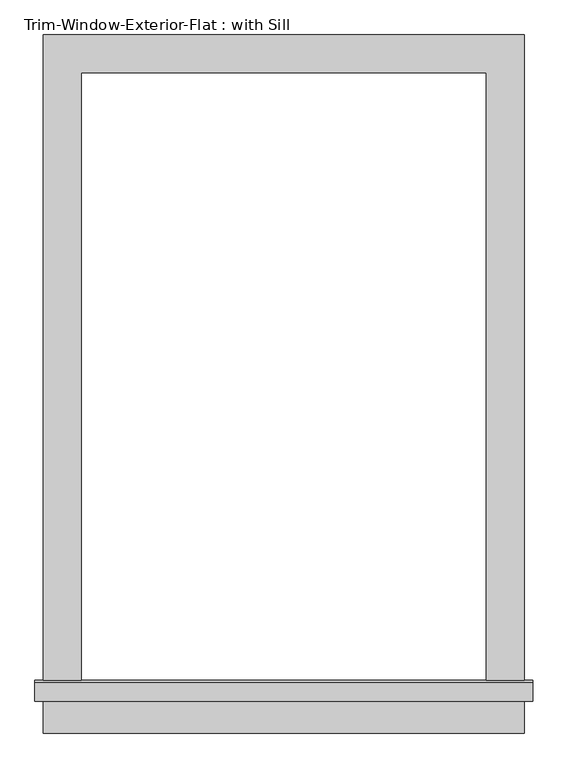
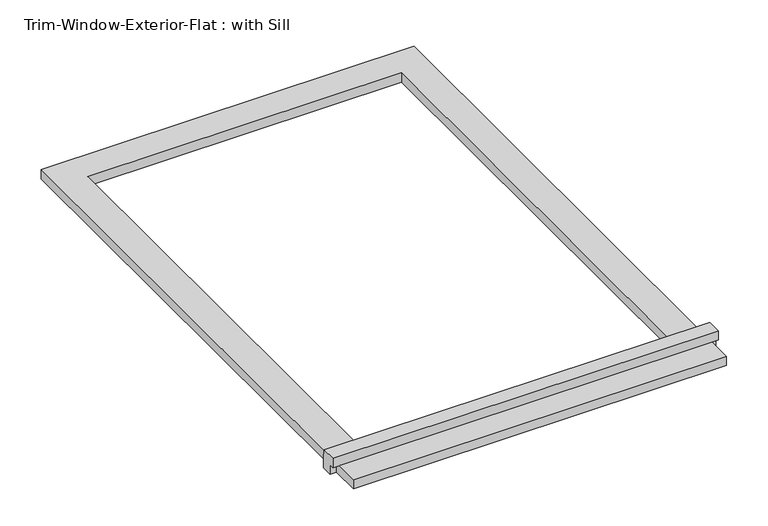
"""IFC4 building model written with IfcOpenShell, lengths in millimetres: proxy geometry, Trim-Window-Exterior-Flat : with Sill."""

from ifc_helpers import new_model, si_unit, frame, origin, origin_with_axes, place, context, project, spatial, polyline, outline, extrude, source, transform, mapped, element, save


def trim_window_exterior_flat_with_sill_a665a915(model_context):
    return source(origin(), model_context, "Body", "SweptSolid", [
        extrude(outline(polyline([(361.95, -936.5823709), (361.95, -993.7323709), (-361.95, -993.7323709), (-361.95, -936.5823709), (361.95, -936.5823709)])), origin_with_axes(), (0.0, 0.0, 1.0), 19.05),
        extrude(outline(polyline([(-946.15, 38.1), (-916.8580645, 38.1), (-914.4, 19.05), (-914.4, 0.0), (-936.5823709, 0.0), (-936.5823709, 19.05), (-946.15, 19.05), (-946.15, 38.1)])), frame((-374.65, 0.0, 0.0), z_axis=(1.0, 0.0, 0.0), x_axis=(0.0, 1.0, 0.0)), (0.0, 0.0, 1.0), 749.3),
        extrude(outline(polyline([(-361.95, 57.15), (361.95, 57.15), (361.95, -914.4), (304.8, -914.4), (304.8, 0.0), (-304.8, 0.0), (-304.8, -914.4), (-361.95, -914.4), (-361.95, 57.15)])), origin_with_axes(), (0.0, 0.0, 1.0), 19.05),
    ])


if __name__ == "__main__":
    model = new_model("IFC4")
    model_context = context("Model", 3, world=origin())
    ifc_project = project(units=[si_unit("LENGTHUNIT", "METRE", prefix="MILLI")], contexts=[model_context])
    site = spatial("IfcSite", under=ifc_project)
    building = spatial("IfcBuilding", under=site)
    placement = place(None, origin())
    trim_window_exterior_flat_with_sill_shape = trim_window_exterior_flat_with_sill_a665a915(model_context)
    element("IfcBuildingElementProxy", 1, Name="Trim-Window-Exterior-Flat : with Sill", ObjectType="Trim-Window-Exterior-Flat : with Sill", at=placement, inside=building, context=model_context, shape_type="MappedRepresentation", body=[
        mapped(trim_window_exterior_flat_with_sill_shape, transform((0.0, 0.0, 0.0), x_axis=(1.0, 0.0, 0.0), y_axis=(0.0, 1.0, 0.0), z_axis=(0.0, 0.0, 1.0))),
    ])
    save(model, "model.ifc")

# Revit data of these elements
# Type "Trim-Window-Exterior-Flat : with Sill"
#   Trim Width = 0' - 2 1/4"
#   Trim Thickness_Picture Frame = 0' - 1 1/4"
#   Trim Thickness_with Sill = 0' - 0 3/4"
#   Sill Thickness = 0' - 1 1/4"
#   Opening Width [instance default] = 2' - 0"
#   Opening Height [instance default] = 3' - 0"
#   Default Elevation = 4' - 0"
#   Sill = yes
#   Picture Frame = no
#   Trim Material [instance default] = none
# Element 1 (IfcBuildingElementProxy, "Trim-Window-Exterior-Flat : with Sill")
#   Trim Material = Clad - White
#   Materials on its faces: "Clad - White"
# Materials
#   "Clad - White": class "Wood", colour RGB 245 245 243, transparency 0, Cost = 0
